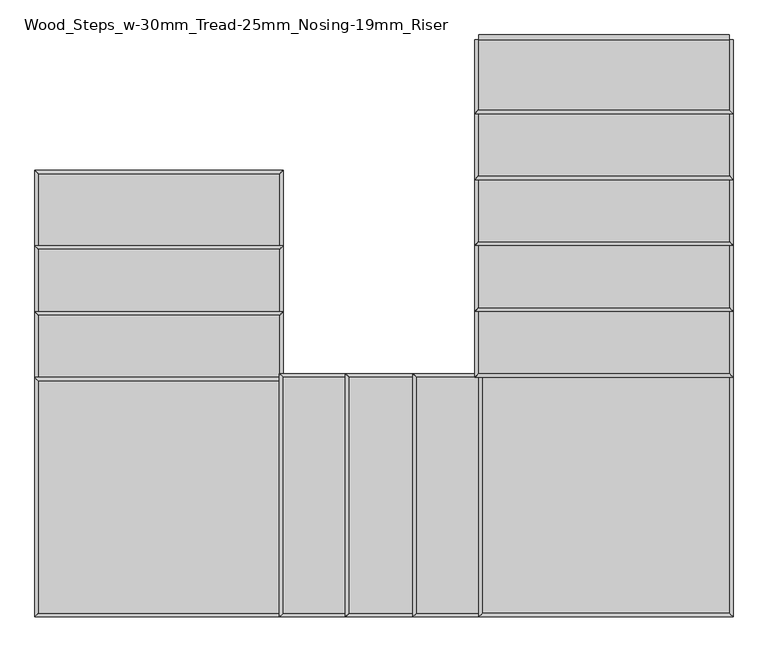
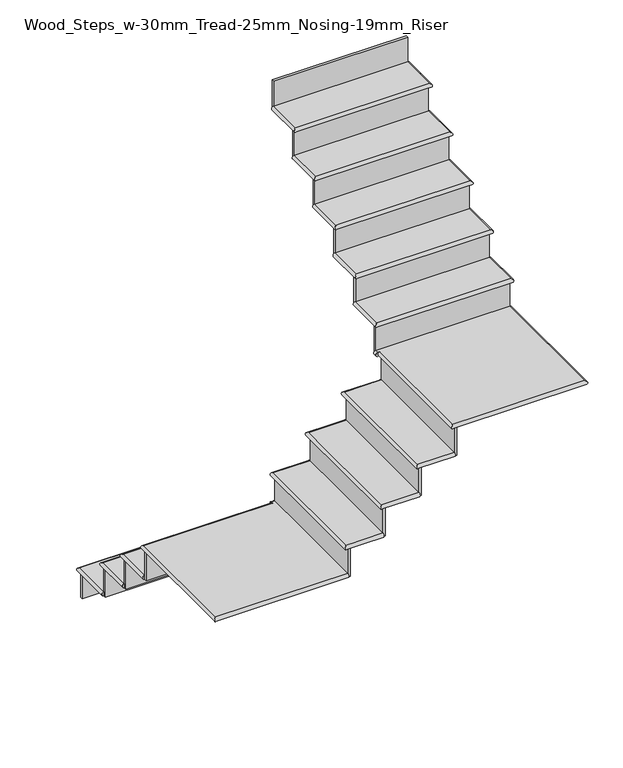
"""IFC4 building model written with IfcOpenShell, lengths in millimetres: stair flight geometry, Wood_Steps_w-30mm_Tread-25mm_Nosing-19mm_Riser."""

from ifc_helpers import new_model, si_unit, frame, origin, place, context, project, spatial, circle_curve, ellipse_curve, faceted_brep, source, transform, mapped, element, save
from ifc_brep_helpers import plane_surface, cylinder_surface, advanced_brep


def wood_steps_w_30mm_tread_25mm_nosing_19mm_riser_e02fc27e(model_context):
    return source(origin(), model_context, "Body", "SolidModel", [
        advanced_brep(
        [(-4339.3477418, 1457.6922428, 187.7142857), (-4339.3477418, 1457.6922428, 217.7142857), (-3412.2477418, 1457.6922428, 217.7142857), (-3412.2477418, 1457.6922428, 187.7142857), (-4339.3477418, 1156.5414829, 217.7142857), (-3412.2477418, 1156.5414829, 217.7142857), (-3412.2477418, 1156.5414829, 187.7142857), (-4339.3477418, 1156.5414829, 187.7142857)],
        [
            (0, 1, ellipse_curve(frame((-4339.3477418, 1457.6922428, 202.7142857), z_axis=(0.7071067811865492, 0.7071067811865458, 0.0), x_axis=(-0.7071067811865458, 0.7071067811865491, 0.0)), 21.2132034, 15.0)),
            (1, 2),
            (2, 3, ellipse_curve(frame((-3412.2477418, 1457.6922428, 202.7142857), z_axis=(-0.7071067811865458, 0.7071067811865492, 0.0), x_axis=(-0.7071067811865492, -0.7071067811865458, 0.0)), 21.2132034, 15.0)),
            (3, 0),
            (4, 5),
            (5, 2),
            (1, 4),
            (6, 7),
            (7, 0),
            (3, 6),
            (4, 7, circle_curve(frame((-4339.3477418, 1156.5414829, 202.7142857), z_axis=(0.0, -1.0, 0.0), x_axis=(1.0, 0.0, 0.0)), 15.0)),
            (6, 5, circle_curve(frame((-3412.2477418, 1156.5414829, 202.7142857), z_axis=(0.0, -1.0, 0.0), x_axis=(-1.0, 0.0, 0.0)), 15.0)),
        ],
        [
            cylinder_surface(frame((-4339.3477418, 1457.6922428, 202.7142857), z_axis=(-1.0, 0.0, 0.0), x_axis=(0.0, -1.0, 0.0)), 15.0),
            plane_surface(frame((-3412.2477418, 1435.5414829, 217.7142857), z_axis=(0.0, 0.0, 1.0), x_axis=(0.0, 1.0, 0.0))),
            plane_surface(frame((-3412.2477418, 1435.5414829, 187.7142857), z_axis=(0.0, 0.0, -1.0), x_axis=(0.0, -1.0, 0.0))),
            plane_surface(frame((-4339.3477418, 1156.5414829, 217.7142857), z_axis=(0.0, -1.0, 0.0), x_axis=(0.0, 0.0, -1.0))),
            cylinder_surface(frame((-4339.3477418, 1156.5414829, 202.7142857), z_axis=(0.0, -1.0, 0.0), x_axis=(1.0, 0.0, 0.0)), 15.0),
            cylinder_surface(frame((-3412.2477418, 1457.6922428, 202.7142857), z_axis=(0.0, 1.0, 0.0), x_axis=(-1.0, 0.0, 0.0)), 15.0),
        ],
        [
            (0, [[1, 2, 3, 4]]),
            (1, [[5, 6, -2, 7]]),
            (2, [[8, 9, -4, 10]]),
            (3, [[-5, 11, -8, 12]]),
            (4, [[-11, -7, -1, -9]]),
            (5, [[-3, -6, -12, -10]]),
        ],
    ),
        faceted_brep([(-4339.3477418, 1447.6922428, 187.7142857), (-4339.3477418, 1447.6922428, 0.0), (-4339.3477418, 1428.6922428, 0.0), (-4339.3477418, 1428.6922428, 187.7142857), (-3412.2477418, 1447.6922428, 187.7142857), (-3412.2477418, 1428.6922428, 187.7142857), (-3412.2477418, 1428.6922428, 0.0), (-3412.2477418, 1447.6922428, 0.0)], [[[0, 1, 2, 3]], [[4, 5, 6, 7]], [[1, 0, 4, 7]], [[2, 1, 7, 6]], [[3, 2, 6, 5]], [[0, 3, 5, 4]]]),
        faceted_brep([(-4339.3477418, 1156.5414829, 405.4285714), (-4339.3477418, 1156.5414829, 187.7142857), (-4339.3477418, 1137.5414829, 187.7142857), (-4339.3477418, 1137.5414829, 405.4285714), (-3412.2477418, 1156.5414829, 405.4285714), (-3412.2477418, 1137.5414829, 405.4285714), (-3412.2477418, 1137.5414829, 187.7142857), (-3412.2477418, 1156.5414829, 187.7142857)], [[[0, 1, 2, 3]], [[4, 5, 6, 7]], [[1, 0, 4, 7]], [[2, 1, 7, 6]], [[3, 2, 6, 5]], [[0, 3, 5, 4]]]),
        advanced_brep(
        [(-4339.3477418, 902.5414829, 435.4285714), (-3412.2477418, 902.5414829, 435.4285714), (-3412.2477418, 1166.5414829, 435.4285714), (-4339.3477418, 1166.5414829, 435.4285714), (-3412.2477418, 902.5414829, 405.4285714), (-4339.3477418, 902.5414829, 405.4285714), (-4339.3477418, 1166.5414829, 405.4285714), (-3412.2477418, 1166.5414829, 405.4285714)],
        [
            (0, 1),
            (1, 2),
            (2, 3),
            (3, 0),
            (4, 5),
            (5, 6),
            (6, 7),
            (7, 4),
            (0, 5, circle_curve(frame((-4339.3477418, 902.5414829, 420.4285714), z_axis=(0.0, -1.0, 0.0), x_axis=(1.0, 0.0, 0.0)), 15.0)),
            (4, 1, circle_curve(frame((-3412.2477418, 902.5414829, 420.4285714), z_axis=(0.0, -1.0, 0.0), x_axis=(-1.0, 0.0, 0.0)), 15.0)),
            (6, 3, ellipse_curve(frame((-4339.3477418, 1166.5414829, 420.4285714), z_axis=(0.7071067811865492, 0.7071067811865458, 0.0), x_axis=(-0.7071067811865458, 0.7071067811865491, 0.0)), 21.2132034, 15.0)),
            (2, 7, ellipse_curve(frame((-3412.2477418, 1166.5414829, 420.4285714), z_axis=(-0.7071067811865458, 0.7071067811865492, 0.0), x_axis=(-0.7071067811865492, -0.7071067811865458, 0.0)), 21.2132034, 15.0)),
        ],
        [
            plane_surface(frame((-3412.2477418, 1435.5414829, 435.4285714), z_axis=(0.0, 0.0, 1.0), x_axis=(0.0, 1.0, 0.0))),
            plane_surface(frame((-3412.2477418, 1435.5414829, 405.4285714), z_axis=(0.0, 0.0, -1.0), x_axis=(0.0, -1.0, 0.0))),
            plane_surface(frame((-4339.3477418, 902.5414829, 435.4285714), z_axis=(0.0, -1.0, 0.0), x_axis=(0.0, 0.0, -1.0))),
            cylinder_surface(frame((-4339.3477418, 1166.5414829, 420.4285714), z_axis=(-1.0, 0.0, 0.0), x_axis=(0.0, -1.0, 0.0)), 15.0),
            cylinder_surface(frame((-4339.3477418, 902.5414829, 420.4285714), z_axis=(0.0, -1.0, 0.0), x_axis=(1.0, 0.0, 0.0)), 15.0),
            cylinder_surface(frame((-3412.2477418, 1166.5414829, 420.4285714), z_axis=(0.0, 1.0, 0.0), x_axis=(-1.0, 0.0, 0.0)), 15.0),
        ],
        [
            (0, [[1, 2, 3, 4]]),
            (1, [[5, 6, 7, 8]]),
            (2, [[-1, 9, -5, 10]]),
            (3, [[11, -3, 12, -7]]),
            (4, [[-9, -4, -11, -6]]),
            (5, [[-12, -2, -10, -8]]),
        ],
    ),
        faceted_brep([(-4339.3477418, 902.5414829, 623.1428571), (-4339.3477418, 902.5414829, 405.4285714), (-4339.3477418, 883.5414829, 405.4285714), (-4339.3477418, 883.5414829, 623.1428571), (-3412.2477418, 902.5414829, 623.1428571), (-3412.2477418, 883.5414829, 623.1428571), (-3412.2477418, 883.5414829, 405.4285714), (-3412.2477418, 902.5414829, 405.4285714)], [[[0, 1, 2, 3]], [[4, 5, 6, 7]], [[1, 0, 4, 7]], [[2, 1, 7, 6]], [[3, 2, 6, 5]], [[0, 3, 5, 4]]]),
        advanced_brep(
        [(-4339.3477418, 648.5414829, 653.1428571), (-3412.2477418, 648.5414829, 653.1428571), (-3412.2477418, 912.5414829, 653.1428571), (-4339.3477418, 912.5414829, 653.1428571), (-3412.2477418, 648.5414829, 623.1428571), (-4339.3477418, 648.5414829, 623.1428571), (-4339.3477418, 912.5414829, 623.1428571), (-3412.2477418, 912.5414829, 623.1428571)],
        [
            (0, 1),
            (1, 2),
            (2, 3),
            (3, 0),
            (4, 5),
            (5, 6),
            (6, 7),
            (7, 4),
            (0, 5, circle_curve(frame((-4339.3477418, 648.5414829, 638.1428571), z_axis=(0.0, -1.0, 0.0), x_axis=(1.0, 0.0, 0.0)), 15.0)),
            (4, 1, circle_curve(frame((-3412.2477418, 648.5414829, 638.1428571), z_axis=(0.0, -1.0, 0.0), x_axis=(-1.0, 0.0, 0.0)), 15.0)),
            (6, 3, ellipse_curve(frame((-4339.3477418, 912.5414829, 638.1428571), z_axis=(0.7071067811865492, 0.7071067811865458, 0.0), x_axis=(-0.7071067811865458, 0.7071067811865491, 0.0)), 21.2132034, 15.0)),
            (2, 7, ellipse_curve(frame((-3412.2477418, 912.5414829, 638.1428571), z_axis=(-0.7071067811865458, 0.7071067811865492, 0.0), x_axis=(-0.7071067811865492, -0.7071067811865458, 0.0)), 21.2132034, 15.0)),
        ],
        [
            plane_surface(frame((-3412.2477418, 1181.5414829, 653.1428571), z_axis=(0.0, 0.0, 1.0), x_axis=(0.0, 1.0, 0.0))),
            plane_surface(frame((-3412.2477418, 1181.5414829, 623.1428571), z_axis=(0.0, 0.0, -1.0), x_axis=(0.0, -1.0, 0.0))),
            plane_surface(frame((-4339.3477418, 648.5414829, 653.1428571), z_axis=(0.0, -1.0, 0.0), x_axis=(0.0, 0.0, -1.0))),
            cylinder_surface(frame((-4339.3477418, 912.5414829, 638.1428571), z_axis=(-1.0, 0.0, 0.0), x_axis=(0.0, -1.0, 0.0)), 15.0),
            cylinder_surface(frame((-4339.3477418, 648.5414829, 638.1428571), z_axis=(0.0, -1.0, 0.0), x_axis=(1.0, 0.0, 0.0)), 15.0),
            cylinder_surface(frame((-3412.2477418, 912.5414829, 638.1428571), z_axis=(0.0, 1.0, 0.0), x_axis=(-1.0, 0.0, 0.0)), 15.0),
        ],
        [
            (0, [[1, 2, 3, 4]]),
            (1, [[5, 6, 7, 8]]),
            (2, [[-1, 9, -5, 10]]),
            (3, [[11, -3, 12, -7]]),
            (4, [[-9, -4, -11, -6]]),
            (5, [[-12, -2, -10, -8]]),
        ],
    ),
        faceted_brep([(-4339.3477418, 648.5414829, 840.8571429), (-4339.3477418, 648.5414829, 623.1428571), (-4339.3477418, 629.5414829, 623.1428571), (-4339.3477418, 629.5414829, 840.8571429), (-3412.2477418, 648.5414829, 840.8571429), (-3412.2477418, 629.5414829, 840.8571429), (-3412.2477418, 629.5414829, 623.1428571), (-3412.2477418, 648.5414829, 623.1428571)], [[[0, 1, 2, 3]], [[4, 5, 6, 7]], [[1, 0, 4, 7]], [[2, 1, 7, 6]], [[3, 2, 6, 5]], [[0, 3, 5, 4]]]),
        advanced_brep(
        [(-3412.2477418, 673.5414829, 870.8571429), (-3412.2477418, 658.5414829, 870.8571429), (-4339.3477418, 658.5414829, 870.8571429), (-4339.3477418, -234.1877572, 870.8571429), (-3387.2477418, -234.1877572, 870.8571429), (-3387.2477418, 673.5414829, 870.8571429), (-3412.2477418, 658.5414829, 840.8571429), (-3412.2477418, 673.5414829, 840.8571429), (-3387.2477418, 673.5414829, 840.8571429), (-3387.2477418, -234.1877572, 840.8571429), (-4339.3477418, -234.1877572, 840.8571429), (-4339.3477418, 658.5414829, 840.8571429)],
        [
            (0, 1),
            (1, 2),
            (2, 3),
            (3, 4),
            (4, 5),
            (5, 0),
            (6, 7),
            (7, 8),
            (8, 9),
            (9, 10),
            (10, 11),
            (11, 6),
            (0, 7, circle_curve(frame((-3412.2477418, 673.5414829, 855.8571429), z_axis=(-1.0, 0.0, 0.0), x_axis=(0.0, -1.0, 0.0)), 15.0)),
            (6, 1, circle_curve(frame((-3412.2477418, 658.5414829, 855.8571429), z_axis=(1.0, 0.0, 0.0), x_axis=(0.0, -1.0, 0.0)), 15.0)),
            (4, 9, circle_curve(frame((-3387.2477418, -234.1877572, 855.8571429), z_axis=(1.0, 0.0, 0.0), x_axis=(0.0, 1.0, 0.0)), 15.0)),
            (8, 5, circle_curve(frame((-3387.2477418, 673.5414829, 855.8571429), z_axis=(1.0, 0.0, 0.0), x_axis=(0.0, -1.0, 0.0)), 15.0)),
            (11, 2, ellipse_curve(frame((-4339.3477418, 658.5414829, 855.8571429), z_axis=(0.7071067811865493, 0.7071067811865456, 0.0), x_axis=(-0.7071067811865457, 0.7071067811865492, 0.0)), 21.2132034, 15.0)),
            (3, 10, ellipse_curve(frame((-4339.3477418, -234.1877572, 855.8571429), z_axis=(0.7071067811865457, -0.7071067811865493, 0.0), x_axis=(0.7071067811865492, 0.7071067811865458, 0.0)), 21.2132034, 15.0)),
        ],
        [
            plane_surface(frame((-3330.1706787, 673.5414829, 870.8571429), z_axis=(0.0, 0.0, 1.0), x_axis=(-1.0, 0.0, 0.0))),
            plane_surface(frame((-3330.1706787, 673.5414829, 840.8571429), z_axis=(0.0, 0.0, -1.0), x_axis=(1.0, 0.0, 0.0))),
            plane_surface(frame((-3412.2477418, 673.5414829, 870.8571429), z_axis=(-1.0, 0.0, 0.0), x_axis=(0.0, 0.0, -1.0))),
            plane_surface(frame((-3387.2477418, -234.1877572, 870.8571429), z_axis=(1.0, 0.0, 0.0), x_axis=(0.0, 0.0, -1.0))),
            cylinder_surface(frame((-4339.3477418, 658.5414829, 855.8571429), z_axis=(-1.0, 0.0, 0.0), x_axis=(0.0, -1.0, 0.0)), 15.0),
            cylinder_surface(frame((-3412.2477418, 673.5414829, 855.8571429), z_axis=(-1.0, 0.0, 0.0), x_axis=(0.0, -1.0, 0.0)), 15.0),
            cylinder_surface(frame((-3387.2477418, -234.1877572, 855.8571429), z_axis=(1.0, 0.0, 0.0), x_axis=(0.0, 1.0, 0.0)), 15.0),
            cylinder_surface(frame((-4339.3477418, -234.1877572, 855.8571429), z_axis=(0.0, -1.0, 0.0), x_axis=(1.0, 0.0, 0.0)), 15.0),
        ],
        [
            (0, [[1, 2, 3, 4, 5, 6]]),
            (1, [[7, 8, 9, 10, 11, 12]]),
            (2, [[-1, 13, -7, 14]]),
            (3, [[-5, 15, -9, 16]]),
            (4, [[17, -2, -14, -12]]),
            (5, [[-13, -6, -16, -8]]),
            (6, [[-15, -4, 18, -10]]),
            (7, [[-18, -3, -17, -11]]),
        ],
    ),
        faceted_brep([(-3387.2477418, -234.1877572, 1058.5714286), (-3387.2477418, -234.1877572, 840.8571429), (-3368.2477418, -234.1877572, 840.8571429), (-3368.2477418, -234.1877572, 1058.5714286), (-3387.2477418, 673.5414829, 1058.5714286), (-3368.2477418, 673.5414829, 1058.5714286), (-3368.2477418, 673.5414829, 840.8571429), (-3387.2477418, 673.5414829, 840.8571429)], [[[0, 1, 2, 3]], [[4, 5, 6, 7]], [[1, 0, 4, 7]], [[2, 1, 7, 6]], [[3, 2, 6, 5]], [[0, 3, 5, 4]]]),
        advanced_brep(
        [(-3133.2477418, -234.1877572, 1088.5714286), (-3133.2477418, 673.5414829, 1088.5714286), (-3397.2477418, 673.5414829, 1088.5714286), (-3397.2477418, -234.1877572, 1088.5714286), (-3133.2477418, 673.5414829, 1058.5714286), (-3133.2477418, -234.1877572, 1058.5714286), (-3397.2477418, -234.1877572, 1058.5714286), (-3397.2477418, 673.5414829, 1058.5714286)],
        [
            (0, 1),
            (1, 2),
            (2, 3),
            (3, 0),
            (4, 5),
            (5, 6),
            (6, 7),
            (7, 4),
            (0, 5, circle_curve(frame((-3133.2477418, -234.1877572, 1073.5714286), z_axis=(1.0, 0.0, 0.0), x_axis=(0.0, 1.0, 0.0)), 15.0)),
            (4, 1, circle_curve(frame((-3133.2477418, 673.5414829, 1073.5714286), z_axis=(1.0, 0.0, 0.0), x_axis=(0.0, -1.0, 0.0)), 15.0)),
            (6, 3, ellipse_curve(frame((-3397.2477418, -234.1877572, 1073.5714286), z_axis=(-0.7071067811865456, 0.7071067811865493, 0.0), x_axis=(-0.7071067811865493, -0.7071067811865457, 0.0)), 21.2132034, 15.0)),
            (2, 7, ellipse_curve(frame((-3397.2477418, 673.5414829, 1073.5714286), z_axis=(-0.7071067811865489, -0.7071067811865462, 0.0), x_axis=(0.7071067811865462, -0.7071067811865488, 0.0)), 21.2132034, 15.0)),
        ],
        [
            plane_surface(frame((-3330.1706787, 673.5414829, 1088.5714286), z_axis=(0.0, 0.0, 1.0), x_axis=(-1.0, 0.0, 0.0))),
            plane_surface(frame((-3330.1706787, 673.5414829, 1058.5714286), z_axis=(0.0, 0.0, -1.0), x_axis=(1.0, 0.0, 0.0))),
            plane_surface(frame((-3133.2477418, -234.1877572, 1088.5714286), z_axis=(1.0, 0.0, 0.0), x_axis=(0.0, 0.0, -1.0))),
            cylinder_surface(frame((-3397.2477418, -234.1877572, 1073.5714286), z_axis=(0.0, -1.0, 0.0), x_axis=(1.0, 0.0, 0.0)), 15.0),
            cylinder_surface(frame((-3133.2477418, -234.1877572, 1073.5714286), z_axis=(1.0, 0.0, 0.0), x_axis=(0.0, 1.0, 0.0)), 15.0),
            cylinder_surface(frame((-3397.2477418, 673.5414829, 1073.5714286), z_axis=(-1.0, 0.0, 0.0), x_axis=(0.0, -1.0, 0.0)), 15.0),
        ],
        [
            (0, [[1, 2, 3, 4]]),
            (1, [[5, 6, 7, 8]]),
            (2, [[-1, 9, -5, 10]]),
            (3, [[11, -3, 12, -7]]),
            (4, [[-9, -4, -11, -6]]),
            (5, [[-12, -2, -10, -8]]),
        ],
    ),
        faceted_brep([(-3133.2477418, -234.1877572, 1276.2857143), (-3133.2477418, -234.1877572, 1058.5714286), (-3114.2477418, -234.1877572, 1058.5714286), (-3114.2477418, -234.1877572, 1276.2857143), (-3133.2477418, 673.5414829, 1276.2857143), (-3114.2477418, 673.5414829, 1276.2857143), (-3114.2477418, 673.5414829, 1058.5714286), (-3133.2477418, 673.5414829, 1058.5714286)], [[[0, 1, 2, 3]], [[4, 5, 6, 7]], [[1, 0, 4, 7]], [[2, 1, 7, 6]], [[3, 2, 6, 5]], [[0, 3, 5, 4]]]),
        advanced_brep(
        [(-2873.3706787, -234.1877572, 1306.2857143), (-2873.3706787, 673.5414829, 1306.2857143), (-3143.2477418, 673.5414829, 1306.2857143), (-3143.2477418, -234.1877572, 1306.2857143), (-2873.3706787, 673.5414829, 1276.2857143), (-2873.3706787, -234.1877572, 1276.2857143), (-3143.2477418, -234.1877572, 1276.2857143), (-3143.2477418, 673.5414829, 1276.2857143)],
        [
            (0, 1),
            (1, 2),
            (2, 3),
            (3, 0),
            (4, 5),
            (5, 6),
            (6, 7),
            (7, 4),
            (0, 5, circle_curve(frame((-2873.3706787, -234.1877572, 1291.2857143), z_axis=(1.0, 0.0, 0.0), x_axis=(0.0, 1.0, 0.0)), 15.0)),
            (4, 1, circle_curve(frame((-2873.3706787, 673.5414829, 1291.2857143), z_axis=(1.0, 0.0, 0.0), x_axis=(0.0, -1.0, 0.0)), 15.0)),
            (6, 3, ellipse_curve(frame((-3143.2477418, -234.1877572, 1291.2857143), z_axis=(-0.7071067811865456, 0.7071067811865493, 0.0), x_axis=(-0.7071067811865493, -0.7071067811865457, 0.0)), 21.2132034, 15.0)),
            (2, 7, ellipse_curve(frame((-3143.2477418, 673.5414829, 1291.2857143), z_axis=(-0.7071067811865489, -0.7071067811865461, 0.0), x_axis=(0.7071067811865461, -0.7071067811865489, 0.0)), 21.2132034, 15.0)),
        ],
        [
            plane_surface(frame((-3330.1706787, 673.5414829, 1306.2857143), z_axis=(0.0, 0.0, 1.0), x_axis=(-1.0, 0.0, 0.0))),
            plane_surface(frame((-3330.1706787, 673.5414829, 1276.2857143), z_axis=(0.0, 0.0, -1.0), x_axis=(1.0, 0.0, 0.0))),
            plane_surface(frame((-2873.3706787, -234.1877572, 1306.2857143), z_axis=(1.0, 0.0, 0.0), x_axis=(0.0, 0.0, -1.0))),
            cylinder_surface(frame((-3143.2477418, -234.1877572, 1291.2857143), z_axis=(0.0, -1.0, 0.0), x_axis=(1.0, 0.0, 0.0)), 15.0),
            cylinder_surface(frame((-2873.3706787, -234.1877572, 1291.2857143), z_axis=(1.0, 0.0, 0.0), x_axis=(0.0, 1.0, 0.0)), 15.0),
            cylinder_surface(frame((-3143.2477418, 673.5414829, 1291.2857143), z_axis=(-1.0, 0.0, 0.0), x_axis=(0.0, -1.0, 0.0)), 15.0),
        ],
        [
            (0, [[1, 2, 3, 4]]),
            (1, [[5, 6, 7, 8]]),
            (2, [[-1, 9, -5, 10]]),
            (3, [[11, -3, 12, -7]]),
            (4, [[-9, -4, -11, -6]]),
            (5, [[-12, -2, -10, -8]]),
        ],
    ),
        faceted_brep([(-2873.3706787, -234.1877572, 1494.0), (-2873.3706787, -234.1877572, 1276.2857143), (-2854.3706787, -234.1877572, 1276.2857143), (-2854.3706787, -234.1877572, 1494.0), (-2873.3706787, 673.5414829, 1494.0), (-2854.3706787, 673.5414829, 1494.0), (-2854.3706787, 673.5414829, 1276.2857143), (-2873.3706787, 673.5414829, 1276.2857143)], [[[0, 1, 2, 3]], [[4, 5, 6, 7]], [[1, 0, 4, 7]], [[2, 1, 7, 6]], [[3, 2, 6, 5]], [[0, 3, 5, 4]]]),
        advanced_brep(
        [(-2619.3706787, -234.1877572, 1524.0), (-2619.3706787, 673.5414829, 1524.0), (-2883.3706787, 673.5414829, 1524.0), (-2883.3706787, -234.1877572, 1524.0), (-2619.3706787, 673.5414829, 1494.0), (-2619.3706787, -234.1877572, 1494.0), (-2883.3706787, -234.1877572, 1494.0), (-2883.3706787, 673.5414829, 1494.0)],
        [
            (0, 1),
            (1, 2),
            (2, 3),
            (3, 0),
            (4, 5),
            (5, 6),
            (6, 7),
            (7, 4),
            (0, 5, circle_curve(frame((-2619.3706787, -234.1877572, 1509.0), z_axis=(1.0, 0.0, 0.0), x_axis=(0.0, 1.0, 0.0)), 15.0)),
            (4, 1, circle_curve(frame((-2619.3706787, 673.5414829, 1509.0), z_axis=(1.0, 0.0, 0.0), x_axis=(0.0, -1.0, 0.0)), 15.0)),
            (6, 3, ellipse_curve(frame((-2883.3706787, -234.1877572, 1509.0), z_axis=(-0.7071067811865456, 0.7071067811865493, 0.0), x_axis=(-0.7071067811865493, -0.7071067811865457, 0.0)), 21.2132034, 15.0)),
            (2, 7, ellipse_curve(frame((-2883.3706787, 673.5414829, 1509.0), z_axis=(-0.7071067811865489, -0.7071067811865461, 0.0), x_axis=(0.7071067811865461, -0.7071067811865489, 0.0)), 21.2132034, 15.0)),
        ],
        [
            plane_surface(frame((-3330.1706787, 673.5414829, 1524.0), z_axis=(0.0, 0.0, 1.0), x_axis=(-1.0, 0.0, 0.0))),
            plane_surface(frame((-3330.1706787, 673.5414829, 1494.0), z_axis=(0.0, 0.0, -1.0), x_axis=(1.0, 0.0, 0.0))),
            plane_surface(frame((-2619.3706787, -234.1877572, 1524.0), z_axis=(1.0, 0.0, 0.0), x_axis=(0.0, 0.0, -1.0))),
            cylinder_surface(frame((-2883.3706787, -234.1877572, 1509.0), z_axis=(0.0, -1.0, 0.0), x_axis=(1.0, 0.0, 0.0)), 15.0),
            cylinder_surface(frame((-2619.3706787, -234.1877572, 1509.0), z_axis=(1.0, 0.0, 0.0), x_axis=(0.0, 1.0, 0.0)), 15.0),
            cylinder_surface(frame((-2883.3706787, 673.5414829, 1509.0), z_axis=(-1.0, 0.0, 0.0), x_axis=(0.0, -1.0, 0.0)), 15.0),
        ],
        [
            (0, [[1, 2, 3, 4]]),
            (1, [[5, 6, 7, 8]]),
            (2, [[-1, 9, -5, 10]]),
            (3, [[11, -3, 12, -7]]),
            (4, [[-9, -4, -11, -6]]),
            (5, [[-12, -2, -10, -8]]),
        ],
    ),
        faceted_brep([(-2619.3706787, -234.1877572, 1711.7142857), (-2619.3706787, -234.1877572, 1494.0), (-2600.3706787, -234.1877572, 1494.0), (-2600.3706787, -234.1877572, 1711.7142857), (-2619.3706787, 673.5414829, 1711.7142857), (-2600.3706787, 673.5414829, 1711.7142857), (-2600.3706787, 673.5414829, 1494.0), (-2619.3706787, 673.5414829, 1494.0)], [[[0, 1, 2, 3]], [[4, 5, 6, 7]], [[1, 0, 4, 7]], [[2, 1, 7, 6]], [[3, 2, 6, 5]], [[0, 3, 5, 4]]]),
        advanced_brep(
        [(-2644.3706787, 673.5414829, 1741.7142857), (-2629.3706787, 673.5414829, 1741.7142857), (-2629.3706787, -234.1877572, 1741.7142857), (-1679.5596772, -234.1877572, 1741.7142857), (-1679.5596772, 698.5414829, 1741.7142857), (-2644.3706787, 698.5414829, 1741.7142857), (-2629.3706787, 673.5414829, 1711.7142857), (-2644.3706787, 673.5414829, 1711.7142857), (-2644.3706787, 698.5414829, 1711.7142857), (-1679.5596772, 698.5414829, 1711.7142857), (-1679.5596772, -234.1877572, 1711.7142857), (-2629.3706787, -234.1877572, 1711.7142857)],
        [
            (0, 1),
            (1, 2),
            (2, 3),
            (3, 4),
            (4, 5),
            (5, 0),
            (6, 7),
            (7, 8),
            (8, 9),
            (9, 10),
            (10, 11),
            (11, 6),
            (0, 7, circle_curve(frame((-2644.3706787, 673.5414829, 1726.7142857), z_axis=(0.0, -1.0, 0.0), x_axis=(1.0, 0.0, 0.0)), 15.0)),
            (6, 1, circle_curve(frame((-2629.3706787, 673.5414829, 1726.7142857), z_axis=(0.0, 1.0, 0.0), x_axis=(1.0, 0.0, 0.0)), 15.0)),
            (4, 9, circle_curve(frame((-1679.5596772, 698.5414829, 1726.7142857), z_axis=(0.0, 1.0, 0.0), x_axis=(-1.0, 0.0, 0.0)), 15.0)),
            (8, 5, circle_curve(frame((-2644.3706787, 698.5414829, 1726.7142857), z_axis=(0.0, 1.0, 0.0), x_axis=(1.0, 0.0, 0.0)), 15.0)),
            (11, 2, ellipse_curve(frame((-2629.3706787, -234.1877572, 1726.7142857), z_axis=(-0.7071067811865457, 0.7071067811865492, 0.0), x_axis=(-0.7071067811865491, -0.7071067811865459, 0.0)), 21.2132034, 15.0)),
            (3, 10, ellipse_curve(frame((-1679.5596772, -234.1877572, 1726.7142857), z_axis=(0.7071067811865491, 0.7071067811865459, 0.0), x_axis=(-0.7071067811865458, 0.7071067811865492, 0.0)), 21.2132034, 15.0)),
        ],
        [
            plane_surface(frame((-2644.3706787, 749.7414829, 1741.7142857), z_axis=(0.0, 0.0, 1.0), x_axis=(0.0, -1.0, 0.0))),
            plane_surface(frame((-2644.3706787, 749.7414829, 1711.7142857), z_axis=(0.0, 0.0, -1.0), x_axis=(0.0, 1.0, 0.0))),
            plane_surface(frame((-2644.3706787, 673.5414829, 1741.7142857), z_axis=(0.0, -1.0, 0.0), x_axis=(0.0, 0.0, -1.0))),
            plane_surface(frame((-1679.5596772, 698.5414829, 1741.7142857), z_axis=(0.0, 1.0, 0.0), x_axis=(0.0, 0.0, -1.0))),
            cylinder_surface(frame((-2629.3706787, -234.1877572, 1726.7142857), z_axis=(0.0, -1.0, 0.0), x_axis=(1.0, 0.0, 0.0)), 15.0),
            cylinder_surface(frame((-2644.3706787, 673.5414829, 1726.7142857), z_axis=(0.0, -1.0, 0.0), x_axis=(1.0, 0.0, 0.0)), 15.0),
            cylinder_surface(frame((-1679.5596772, 698.5414829, 1726.7142857), z_axis=(0.0, 1.0, 0.0), x_axis=(-1.0, 0.0, 0.0)), 15.0),
            cylinder_surface(frame((-1679.5596772, -234.1877572, 1726.7142857), z_axis=(1.0, 0.0, 0.0), x_axis=(0.0, 1.0, 0.0)), 15.0),
        ],
        [
            (0, [[1, 2, 3, 4, 5, 6]]),
            (1, [[7, 8, 9, 10, 11, 12]]),
            (2, [[-1, 13, -7, 14]]),
            (3, [[-5, 15, -9, 16]]),
            (4, [[17, -2, -14, -12]]),
            (5, [[-13, -6, -16, -8]]),
            (6, [[-15, -4, 18, -10]]),
            (7, [[-18, -3, -17, -11]]),
        ],
    ),
        faceted_brep([(-1679.5596772, 698.5414829, 1929.4285714), (-1679.5596772, 698.5414829, 1711.7142857), (-1679.5596772, 717.5414829, 1711.7142857), (-1679.5596772, 717.5414829, 1929.4285714), (-2644.3706787, 698.5414829, 1929.4285714), (-2644.3706787, 717.5414829, 1929.4285714), (-2644.3706787, 717.5414829, 1711.7142857), (-2644.3706787, 698.5414829, 1711.7142857)], [[[0, 1, 2, 3]], [[4, 5, 6, 7]], [[1, 0, 4, 7]], [[2, 1, 7, 6]], [[3, 2, 6, 5]], [[0, 3, 5, 4]]]),
        advanced_brep(
        [(-1679.5596772, 952.5414829, 1959.4285714), (-2644.3706787, 952.5414829, 1959.4285714), (-2644.3706787, 688.5414829, 1959.4285714), (-1679.5596772, 688.5414829, 1959.4285714), (-2644.3706787, 952.5414829, 1929.4285714), (-1679.5596772, 952.5414829, 1929.4285714), (-1679.5596772, 688.5414829, 1929.4285714), (-2644.3706787, 688.5414829, 1929.4285714)],
        [
            (0, 1),
            (1, 2),
            (2, 3),
            (3, 0),
            (4, 5),
            (5, 6),
            (6, 7),
            (7, 4),
            (0, 5, circle_curve(frame((-1679.5596772, 952.5414829, 1944.4285714), z_axis=(0.0, 1.0, 0.0), x_axis=(-1.0, 0.0, 0.0)), 15.0)),
            (4, 1, circle_curve(frame((-2644.3706787, 952.5414829, 1944.4285714), z_axis=(0.0, 1.0, 0.0), x_axis=(1.0, 0.0, 0.0)), 15.0)),
            (6, 3, ellipse_curve(frame((-1679.5596772, 688.5414829, 1944.4285714), z_axis=(-0.7071067811865491, -0.7071067811865459, 0.0), x_axis=(0.7071067811865458, -0.7071067811865491, 0.0)), 21.2132034, 15.0)),
            (2, 7, ellipse_curve(frame((-2644.3706787, 688.5414829, 1944.4285714), z_axis=(0.7071067811865458, -0.7071067811865491, 0.0), x_axis=(0.7071067811865492, 0.7071067811865457, 0.0)), 21.2132034, 15.0)),
        ],
        [
            plane_surface(frame((-2644.3706787, 749.7414829, 1959.4285714), z_axis=(0.0, 0.0, 1.0), x_axis=(0.0, -1.0, 0.0))),
            plane_surface(frame((-2644.3706787, 749.7414829, 1929.4285714), z_axis=(0.0, 0.0, -1.0), x_axis=(0.0, 1.0, 0.0))),
            plane_surface(frame((-1679.5596772, 952.5414829, 1959.4285714), z_axis=(0.0, 1.0, 0.0), x_axis=(0.0, 0.0, -1.0))),
            cylinder_surface(frame((-1679.5596772, 688.5414829, 1944.4285714), z_axis=(1.0, 0.0, 0.0), x_axis=(0.0, 1.0, 0.0)), 15.0),
            cylinder_surface(frame((-1679.5596772, 952.5414829, 1944.4285714), z_axis=(0.0, 1.0, 0.0), x_axis=(-1.0, 0.0, 0.0)), 15.0),
            cylinder_surface(frame((-2644.3706787, 688.5414829, 1944.4285714), z_axis=(0.0, -1.0, 0.0), x_axis=(1.0, 0.0, 0.0)), 15.0),
        ],
        [
            (0, [[1, 2, 3, 4]]),
            (1, [[5, 6, 7, 8]]),
            (2, [[-1, 9, -5, 10]]),
            (3, [[11, -3, 12, -7]]),
            (4, [[-9, -4, -11, -6]]),
            (5, [[-12, -2, -10, -8]]),
        ],
    ),
        faceted_brep([(-1679.5596772, 952.5414829, 2147.1428571), (-1679.5596772, 952.5414829, 1929.4285714), (-1679.5596772, 971.5414829, 1929.4285714), (-1679.5596772, 971.5414829, 2147.1428571), (-2644.3706787, 952.5414829, 2147.1428571), (-2644.3706787, 971.5414829, 2147.1428571), (-2644.3706787, 971.5414829, 1929.4285714), (-2644.3706787, 952.5414829, 1929.4285714)], [[[0, 1, 2, 3]], [[4, 5, 6, 7]], [[1, 0, 4, 7]], [[2, 1, 7, 6]], [[3, 2, 6, 5]], [[0, 3, 5, 4]]]),
        advanced_brep(
        [(-1679.5596772, 1206.5414829, 2177.1428571), (-2644.3706787, 1206.5414829, 2177.1428571), (-2644.3706787, 942.5414829, 2177.1428571), (-1679.5596772, 942.5414829, 2177.1428571), (-2644.3706787, 1206.5414829, 2147.1428571), (-1679.5596772, 1206.5414829, 2147.1428571), (-1679.5596772, 942.5414829, 2147.1428571), (-2644.3706787, 942.5414829, 2147.1428571)],
        [
            (0, 1),
            (1, 2),
            (2, 3),
            (3, 0),
            (4, 5),
            (5, 6),
            (6, 7),
            (7, 4),
            (0, 5, circle_curve(frame((-1679.5596772, 1206.5414829, 2162.1428571), z_axis=(0.0, 1.0, 0.0), x_axis=(-1.0, 0.0, 0.0)), 15.0)),
            (4, 1, circle_curve(frame((-2644.3706787, 1206.5414829, 2162.1428571), z_axis=(0.0, 1.0, 0.0), x_axis=(1.0, 0.0, 0.0)), 15.0)),
            (6, 3, ellipse_curve(frame((-1679.5596772, 942.5414829, 2162.1428571), z_axis=(-0.7071067811865491, -0.7071067811865459, 0.0), x_axis=(0.7071067811865458, -0.7071067811865491, 0.0)), 21.2132034, 15.0)),
            (2, 7, ellipse_curve(frame((-2644.3706787, 942.5414829, 2162.1428571), z_axis=(0.7071067811865458, -0.7071067811865491, 0.0), x_axis=(0.7071067811865492, 0.7071067811865457, 0.0)), 21.2132034, 15.0)),
        ],
        [
            plane_surface(frame((-2644.3706787, 1003.7414829, 2177.1428571), z_axis=(0.0, 0.0, 1.0), x_axis=(0.0, -1.0, 0.0))),
            plane_surface(frame((-2644.3706787, 1003.7414829, 2147.1428571), z_axis=(0.0, 0.0, -1.0), x_axis=(0.0, 1.0, 0.0))),
            plane_surface(frame((-1679.5596772, 1206.5414829, 2177.1428571), z_axis=(0.0, 1.0, 0.0), x_axis=(0.0, 0.0, -1.0))),
            cylinder_surface(frame((-1679.5596772, 942.5414829, 2162.1428571), z_axis=(1.0, 0.0, 0.0), x_axis=(0.0, 1.0, 0.0)), 15.0),
            cylinder_surface(frame((-1679.5596772, 1206.5414829, 2162.1428571), z_axis=(0.0, 1.0, 0.0), x_axis=(-1.0, 0.0, 0.0)), 15.0),
            cylinder_surface(frame((-2644.3706787, 942.5414829, 2162.1428571), z_axis=(0.0, -1.0, 0.0), x_axis=(1.0, 0.0, 0.0)), 15.0),
        ],
        [
            (0, [[1, 2, 3, 4]]),
            (1, [[5, 6, 7, 8]]),
            (2, [[-1, 9, -5, 10]]),
            (3, [[11, -3, 12, -7]]),
            (4, [[-9, -4, -11, -6]]),
            (5, [[-12, -2, -10, -8]]),
        ],
    ),
        faceted_brep([(-1679.5596772, 1206.5414829, 2364.8571429), (-1679.5596772, 1206.5414829, 2147.1428571), (-1679.5596772, 1225.5414829, 2147.1428571), (-1679.5596772, 1225.5414829, 2364.8571429), (-2644.3706787, 1206.5414829, 2364.8571429), (-2644.3706787, 1225.5414829, 2364.8571429), (-2644.3706787, 1225.5414829, 2147.1428571), (-2644.3706787, 1206.5414829, 2147.1428571)], [[[0, 1, 2, 3]], [[4, 5, 6, 7]], [[1, 0, 4, 7]], [[2, 1, 7, 6]], [[3, 2, 6, 5]], [[0, 3, 5, 4]]]),
        advanced_brep(
        [(-1679.5596772, 1460.5414829, 2394.8571429), (-2644.3706787, 1460.5414829, 2394.8571429), (-2644.3706787, 1196.5414829, 2394.8571429), (-1679.5596772, 1196.5414829, 2394.8571429), (-2644.3706787, 1460.5414829, 2364.8571429), (-1679.5596772, 1460.5414829, 2364.8571429), (-1679.5596772, 1196.5414829, 2364.8571429), (-2644.3706787, 1196.5414829, 2364.8571429)],
        [
            (0, 1),
            (1, 2),
            (2, 3),
            (3, 0),
            (4, 5),
            (5, 6),
            (6, 7),
            (7, 4),
            (0, 5, circle_curve(frame((-1679.5596772, 1460.5414829, 2379.8571429), z_axis=(0.0, 1.0, 0.0), x_axis=(-1.0, 0.0, 0.0)), 15.0)),
            (4, 1, circle_curve(frame((-2644.3706787, 1460.5414829, 2379.8571429), z_axis=(0.0, 1.0, 0.0), x_axis=(1.0, 0.0, 0.0)), 15.0)),
            (6, 3, ellipse_curve(frame((-1679.5596772, 1196.5414829, 2379.8571429), z_axis=(-0.7071067811865491, -0.7071067811865459, 0.0), x_axis=(0.7071067811865458, -0.7071067811865491, 0.0)), 21.2132034, 15.0)),
            (2, 7, ellipse_curve(frame((-2644.3706787, 1196.5414829, 2379.8571429), z_axis=(0.7071067811865458, -0.7071067811865491, 0.0), x_axis=(0.7071067811865492, 0.7071067811865457, 0.0)), 21.2132034, 15.0)),
        ],
        [
            plane_surface(frame((-2644.3706787, 1257.7414829, 2394.8571429), z_axis=(0.0, 0.0, 1.0), x_axis=(0.0, -1.0, 0.0))),
            plane_surface(frame((-2644.3706787, 1257.7414829, 2364.8571429), z_axis=(0.0, 0.0, -1.0), x_axis=(0.0, 1.0, 0.0))),
            plane_surface(frame((-1679.5596772, 1460.5414829, 2394.8571429), z_axis=(0.0, 1.0, 0.0), x_axis=(0.0, 0.0, -1.0))),
            cylinder_surface(frame((-1679.5596772, 1196.5414829, 2379.8571429), z_axis=(1.0, 0.0, 0.0), x_axis=(0.0, 1.0, 0.0)), 15.0),
            cylinder_surface(frame((-1679.5596772, 1460.5414829, 2379.8571429), z_axis=(0.0, 1.0, 0.0), x_axis=(-1.0, 0.0, 0.0)), 15.0),
            cylinder_surface(frame((-2644.3706787, 1196.5414829, 2379.8571429), z_axis=(0.0, -1.0, 0.0), x_axis=(1.0, 0.0, 0.0)), 15.0),
        ],
        [
            (0, [[1, 2, 3, 4]]),
            (1, [[5, 6, 7, 8]]),
            (2, [[-1, 9, -5, 10]]),
            (3, [[11, -3, 12, -7]]),
            (4, [[-9, -4, -11, -6]]),
            (5, [[-12, -2, -10, -8]]),
        ],
    ),
        faceted_brep([(-1679.5596772, 1460.5414829, 2582.5714286), (-1679.5596772, 1460.5414829, 2364.8571429), (-1679.5596772, 1479.5414829, 2364.8571429), (-1679.5596772, 1479.5414829, 2582.5714286), (-2644.3706787, 1460.5414829, 2582.5714286), (-2644.3706787, 1479.5414829, 2582.5714286), (-2644.3706787, 1479.5414829, 2364.8571429), (-2644.3706787, 1460.5414829, 2364.8571429)], [[[0, 1, 2, 3]], [[4, 5, 6, 7]], [[1, 0, 4, 7]], [[2, 1, 7, 6]], [[3, 2, 6, 5]], [[0, 3, 5, 4]]]),
        advanced_brep(
        [(-1679.5596772, 1714.5414829, 2612.5714286), (-2644.3706787, 1714.5414829, 2612.5714286), (-2644.3706787, 1450.5414829, 2612.5714286), (-1679.5596772, 1450.5414829, 2612.5714286), (-2644.3706787, 1714.5414829, 2582.5714286), (-1679.5596772, 1714.5414829, 2582.5714286), (-1679.5596772, 1450.5414829, 2582.5714286), (-2644.3706787, 1450.5414829, 2582.5714286)],
        [
            (0, 1),
            (1, 2),
            (2, 3),
            (3, 0),
            (4, 5),
            (5, 6),
            (6, 7),
            (7, 4),
            (0, 5, circle_curve(frame((-1679.5596772, 1714.5414829, 2597.5714286), z_axis=(0.0, 1.0, 0.0), x_axis=(-1.0, 0.0, 0.0)), 15.0)),
            (4, 1, circle_curve(frame((-2644.3706787, 1714.5414829, 2597.5714286), z_axis=(0.0, 1.0, 0.0), x_axis=(1.0, 0.0, 0.0)), 15.0)),
            (6, 3, ellipse_curve(frame((-1679.5596772, 1450.5414829, 2597.5714286), z_axis=(-0.7071067811865491, -0.7071067811865459, 0.0), x_axis=(0.7071067811865458, -0.7071067811865491, 0.0)), 21.2132034, 15.0)),
            (2, 7, ellipse_curve(frame((-2644.3706787, 1450.5414829, 2597.5714286), z_axis=(0.7071067811865458, -0.7071067811865491, 0.0), x_axis=(0.7071067811865492, 0.7071067811865457, 0.0)), 21.2132034, 15.0)),
        ],
        [
            plane_surface(frame((-2644.3706787, 1511.7414829, 2612.5714286), z_axis=(0.0, 0.0, 1.0), x_axis=(0.0, -1.0, 0.0))),
            plane_surface(frame((-2644.3706787, 1511.7414829, 2582.5714286), z_axis=(0.0, 0.0, -1.0), x_axis=(0.0, 1.0, 0.0))),
            plane_surface(frame((-1679.5596772, 1714.5414829, 2612.5714286), z_axis=(0.0, 1.0, 0.0), x_axis=(0.0, 0.0, -1.0))),
            cylinder_surface(frame((-1679.5596772, 1450.5414829, 2597.5714286), z_axis=(1.0, 0.0, 0.0), x_axis=(0.0, 1.0, 0.0)), 15.0),
            cylinder_surface(frame((-1679.5596772, 1714.5414829, 2597.5714286), z_axis=(0.0, 1.0, 0.0), x_axis=(-1.0, 0.0, 0.0)), 15.0),
            cylinder_surface(frame((-2644.3706787, 1450.5414829, 2597.5714286), z_axis=(0.0, -1.0, 0.0), x_axis=(1.0, 0.0, 0.0)), 15.0),
        ],
        [
            (0, [[1, 2, 3, 4]]),
            (1, [[5, 6, 7, 8]]),
            (2, [[-1, 9, -5, 10]]),
            (3, [[11, -3, 12, -7]]),
            (4, [[-9, -4, -11, -6]]),
            (5, [[-12, -2, -10, -8]]),
        ],
    ),
        faceted_brep([(-1679.5596772, 1973.6214829, 3018.0), (-1679.5596772, 1973.6214829, 2800.2857143), (-1679.5596772, 1992.6214829, 2800.2857143), (-1679.5596772, 1992.6214829, 3018.0), (-2644.3706787, 1973.6214829, 3018.0), (-2644.3706787, 1992.6214829, 3018.0), (-2644.3706787, 1992.6214829, 2800.2857143), (-2644.3706787, 1973.6214829, 2800.2857143)], [[[0, 1, 2, 3]], [[4, 5, 6, 7]], [[1, 0, 4, 7]], [[2, 1, 7, 6]], [[3, 2, 6, 5]], [[0, 3, 5, 4]]]),
        faceted_brep([(-1679.5596772, 1714.5414829, 2800.2857143), (-1679.5596772, 1714.5414829, 2582.5714286), (-1679.5596772, 1733.5414829, 2582.5714286), (-1679.5596772, 1733.5414829, 2800.2857143), (-2644.3706787, 1714.5414829, 2800.2857143), (-2644.3706787, 1733.5414829, 2800.2857143), (-2644.3706787, 1733.5414829, 2582.5714286), (-2644.3706787, 1714.5414829, 2582.5714286)], [[[0, 1, 2, 3]], [[4, 5, 6, 7]], [[1, 0, 4, 7]], [[2, 1, 7, 6]], [[3, 2, 6, 5]], [[0, 3, 5, 4]]]),
        advanced_brep(
        [(-1679.5596772, 1973.6214829, 2830.2857143), (-2644.3706787, 1973.6214829, 2830.2857143), (-2644.3706787, 1704.5414829, 2830.2857143), (-1679.5596772, 1704.5414829, 2830.2857143), (-2644.3706787, 1973.6214829, 2800.2857143), (-1679.5596772, 1973.6214829, 2800.2857143), (-1679.5596772, 1704.5414829, 2800.2857143), (-2644.3706787, 1704.5414829, 2800.2857143)],
        [
            (0, 1),
            (1, 2),
            (2, 3),
            (3, 0),
            (4, 5),
            (5, 6),
            (6, 7),
            (7, 4),
            (0, 5, circle_curve(frame((-1679.5596772, 1973.6214829, 2815.2857143), z_axis=(0.0, 1.0, 0.0), x_axis=(-1.0, 0.0, 0.0)), 15.0)),
            (4, 1, circle_curve(frame((-2644.3706787, 1973.6214829, 2815.2857143), z_axis=(0.0, 1.0, 0.0), x_axis=(1.0, 0.0, 0.0)), 15.0)),
            (3, 6, ellipse_curve(frame((-1679.5596772, 1704.5414829, 2815.2857143), z_axis=(0.7071067811865492, 0.7071067811865458, 0.0), x_axis=(-0.7071067811865457, 0.7071067811865492, 0.0)), 21.2132034, 15.0)),
            (2, 7, ellipse_curve(frame((-2644.3706787, 1704.5414829, 2815.2857143), z_axis=(0.7071067811865457, -0.7071067811865492, 0.0), x_axis=(0.7071067811865493, 0.7071067811865457, 0.0)), 21.2132034, 15.0)),
        ],
        [
            plane_surface(frame((-2644.3706787, 749.7414829, 2830.2857143), z_axis=(0.0, 0.0, 1.0), x_axis=(0.0, -1.0, 0.0))),
            plane_surface(frame((-2644.3706787, 749.7414829, 2800.2857143), z_axis=(0.0, 0.0, -1.0), x_axis=(0.0, 1.0, 0.0))),
            plane_surface(frame((-1679.5596772, 1973.6214829, 2830.2857143), z_axis=(0.0, 1.0, 0.0), x_axis=(0.0, 0.0, -1.0))),
            cylinder_surface(frame((-1679.5596772, 1973.6214829, 2815.2857143), z_axis=(0.0, 1.0, 0.0), x_axis=(-1.0, 0.0, 0.0)), 15.0),
            cylinder_surface(frame((-1679.5596772, 1704.5414829, 2815.2857143), z_axis=(1.0, 0.0, 0.0), x_axis=(0.0, 1.0, 0.0)), 15.0),
            cylinder_surface(frame((-2644.3706787, 1704.5414829, 2815.2857143), z_axis=(0.0, -1.0, 0.0), x_axis=(1.0, 0.0, 0.0)), 15.0),
        ],
        [
            (0, [[1, 2, 3, 4]]),
            (1, [[5, 6, 7, 8]]),
            (2, [[-1, 9, -5, 10]]),
            (3, [[-9, -4, 11, -6]]),
            (4, [[-11, -3, 12, -7]]),
            (5, [[-12, -2, -10, -8]]),
        ],
    ),
    ])


if __name__ == "__main__":
    model = new_model("IFC4")
    model_context = context("Model", 3, world=origin())
    ifc_project = project(units=[si_unit("LENGTHUNIT", "METRE", prefix="MILLI")], contexts=[model_context])
    site = spatial("IfcSite", under=ifc_project)
    building = spatial("IfcBuilding", under=site)
    placement = place(None, origin())
    wood_steps_w_30mm_tread_25mm_nosing_19mm_riser_shape = wood_steps_w_30mm_tread_25mm_nosing_19mm_riser_e02fc27e(model_context)
    element("IfcStairFlight", 1, ObjectType="Wood_Steps_w-30mm_Tread-25mm_Nosing-19mm_Riser", at=placement, inside=building, context=model_context, shape_type="MappedRepresentation", body=[
        mapped(wood_steps_w_30mm_tread_25mm_nosing_19mm_riser_shape, transform((0.0, 0.0, 0.0), x_axis=(1.0, 0.0, 0.0), y_axis=(0.0, 1.0, 0.0), z_axis=(0.0, 0.0, 1.0))),
    ])
    save(model, "model.ifc")

# Revit data of these elements
# Element 1 (IfcStairFlight, "Wood_Steps_w-30mm_Tread-25mm_Nosing-19mm_Riser")
#   Materials on its faces: "Cherry", "Wood"
# Materials
#   "Cherry": class "Wood", colour RGB 226 177 128, transparency 0, Description = "Prunus Serotina", Cost = 0
#   "Wood": class "Wood", colour RGB 212 179 113, transparency 0, Description = "Generic wood", Cost = 0
